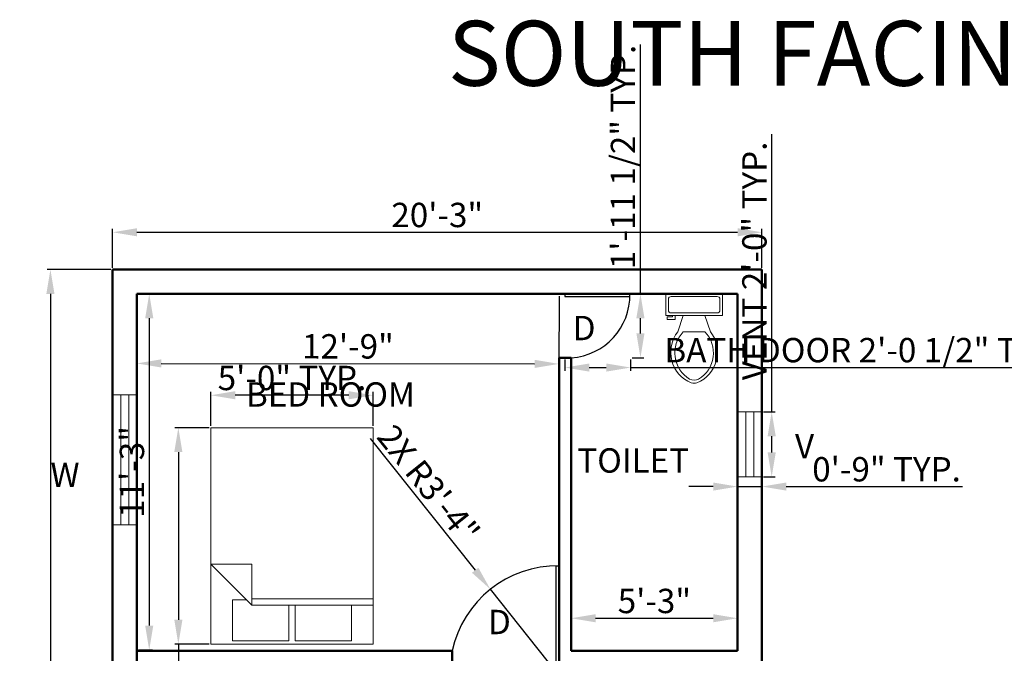
# Model space of a CAD drawing. Units: inches. Extents: x 1802 to 2621, y 1038 to 1686.
# Tile 3 of 5: x 1841 to 2205, y 1452 to 1686. Entities that reach past the tile are written whole.
import ezdxf

# ---------------------------------------------------------------- set-up
doc = ezdxf.new("R2010")
doc.units = ezdxf.units.IN
for name, color, linetype, lineweight in [('A-ANNO-DIMS', 2, 'Continuous', 18), ('A-ANNO-TEXT', 7, 'Continuous', 18), ('A-AREA-IDEN', 7, 'Continuous', 25), ('A-DOOR', 3, 'Continuous', 25), ('A-FLOR-FIXT', 9, 'Continuous', 18), ('A-FURN', 8, 'Continuous', 18), ('A-GLAZ', 4, 'Continuous', 18), ('A-WALL', 7, 'Continuous', 50)]:
    doc.layers.add(name, color=color, linetype=linetype, lineweight=lineweight)
doc.styles.get("Standard").update_dxf_attribs({"font": 'arial.ttf'})
doc.dimstyles.new('ISO-25', dxfattribs={"dimtxt": 9, "dimasz": 9, "dimexe": 1.25, "dimexo": 0.625, "dimtad": 1, "dimdec": 1, "dimrnd": 9, "dimlunit": 3, "dimtxsty": 'Standard', "dimcen": 2.5, "dimadec": 0, "dimazin": 0, "dimtfac": 1, "dimtdec": 1, "dimtmove": 0, "dimatfit": 3, "dimfxl": 1, "dimarcsym": 0})

# ---------------------------------------------------------------- blocks, each defined once
blk = doc.blocks.new('*D1')
at = {"layer": 'A-ANNO-DIMS', "color": 0, "lineweight": -2, "transparency": 16777216}
for p, q in [((1884.73, 1583.93), (1884.7, 1557.61)), ((2040.73, 1583.74), (2040.7, 1557.42)), ((1893.7, 1558.85), (2031.7, 1558.68))]:
    blk.add_line(p, q, dxfattribs=at)
at = {"layer": 'A-ANNO-DIMS', "color": 0, "transparency": 16777216}
for points in [[(1893.7, 1560.35), (1893.7, 1557.35), (1884.7, 1558.86)], [(2031.7, 1560.18), (2031.7, 1557.18), (2040.7, 1558.67)]]:
    blk.add_solid(points, dxfattribs=at)
at = {"layer": 'Defpoints', "color": 0, "transparency": 16777216}
for p in [(1884.73, 1584.56), (2040.73, 1584.37), (2040.7, 1558.67)]:
    blk.add_point(p, dxfattribs=at)
at = {"layer": 'A-ANNO-DIMS', "color": 0, "transparency": 16777216, "insert": (1962.71, 1563.99), "char_height": 9, "attachment_point": 5, "rotation": 359.9308}
blk.add_mtext('12\'-9"', dxfattribs=at)
blk = doc.blocks.new('*D2')
at = {"layer": 'A-ANNO-DIMS', "color": 0, "lineweight": -2, "transparency": 16777216}
for p, q in [((1885.35, 1584.56), (1890.53, 1584.56)), ((1889.28, 1575.56), (1889.28, 1461.93)), ((1885.35, 1452.93), (1890.53, 1452.93))]:
    blk.add_line(p, q, dxfattribs=at)
at = {"layer": 'A-ANNO-DIMS', "color": 0, "transparency": 16777216}
for points in [[(1887.78, 1575.56), (1890.78, 1575.56), (1889.28, 1584.56)], [(1887.78, 1461.93), (1890.78, 1461.93), (1889.28, 1452.93)]]:
    blk.add_solid(points, dxfattribs=at)
at = {"layer": 'Defpoints', "color": 0, "transparency": 16777216}
for p in [(1884.73, 1584.56), (1884.73, 1452.93), (1889.28, 1452.93)]:
    blk.add_point(p, dxfattribs=at)
at = {"layer": 'A-ANNO-DIMS', "color": 0, "transparency": 16777216, "insert": (1884.06, 1518.75), "char_height": 9, "attachment_point": 5, "rotation": 90}
blk.add_mtext('11\'-3"', dxfattribs=at)
blk = doc.blocks.new('*D3')
at = {"layer": 'A-ANNO-DIMS', "color": 0, "lineweight": -2, "transparency": 16777216}
for p, q in [((1875.73, 1594.18), (1875.73, 1608.58)), ((2115.73, 1594.18), (2115.73, 1608.58)), ((1884.73, 1607.33), (2106.73, 1607.33))]:
    blk.add_line(p, q, dxfattribs=at)
at = {"layer": 'A-ANNO-DIMS', "color": 0, "transparency": 16777216}
for points in [[(1884.73, 1608.83), (1884.73, 1605.83), (1875.73, 1607.33)], [(2106.73, 1608.83), (2106.73, 1605.83), (2115.73, 1607.33)]]:
    blk.add_solid(points, dxfattribs=at)
at = {"layer": 'Defpoints', "color": 0, "transparency": 16777216}
for p in [(2115.73, 1607.33), (1875.73, 1593.56), (2115.73, 1593.56)]:
    blk.add_point(p, dxfattribs=at)
at = {"layer": 'A-ANNO-DIMS', "color": 0, "transparency": 16777216, "insert": (1995.73, 1612.56), "char_height": 9, "attachment_point": 5}
blk.add_mtext('20\'-3"', dxfattribs=at)
blk = doc.blocks.new('*D4')
at = {"layer": 'A-ANNO-DIMS', "color": 0, "lineweight": -2, "transparency": 16777216}
for p, q in [((1875.1, 1593.56), (1851.51, 1593.56)), ((1852.76, 1584.56), (1852.76, 1122.56)), ((1875.1, 1113.56), (1851.51, 1113.56))]:
    blk.add_line(p, q, dxfattribs=at)
at = {"layer": 'A-ANNO-DIMS', "color": 0, "transparency": 16777216}
for points in [[(1851.26, 1584.56), (1854.26, 1584.56), (1852.76, 1593.56)], [(1851.26, 1122.56), (1854.26, 1122.56), (1852.76, 1113.56)]]:
    blk.add_solid(points, dxfattribs=at)
at = {"layer": 'Defpoints', "color": 0, "transparency": 16777216}
for p in [(1875.73, 1593.56), (1852.76, 1113.56), (1875.73, 1113.56)]:
    blk.add_point(p, dxfattribs=at)
at = {"layer": 'A-ANNO-DIMS', "color": 0, "transparency": 16777216, "insert": (1847.54, 1353.56), "char_height": 9, "attachment_point": 5, "rotation": 90}
blk.add_mtext('39\'-9"', dxfattribs=at)
blk = doc.blocks.new('*D5')
at = {"layer": 'A-ANNO-DIMS', "color": 0, "lineweight": -2, "transparency": 16777216}
for p, q in [((2045.23, 1453.18), (2045.23, 1465.91)), ((2054.23, 1464.66), (2097.73, 1464.66)), ((2106.73, 1453.18), (2106.73, 1465.91))]:
    blk.add_line(p, q, dxfattribs=at)
at = {"layer": 'A-ANNO-DIMS', "color": 0, "transparency": 16777216}
for points in [[(2054.23, 1466.16), (2054.23, 1463.16), (2045.23, 1464.66)], [(2097.73, 1466.16), (2097.73, 1463.16), (2106.73, 1464.66)]]:
    blk.add_solid(points, dxfattribs=at)
at = {"layer": 'Defpoints', "color": 0, "transparency": 16777216}
for p in [(2106.73, 1464.66), (2045.23, 1452.56), (2106.73, 1452.56)]:
    blk.add_point(p, dxfattribs=at)
at = {"layer": 'A-ANNO-DIMS', "color": 0, "transparency": 16777216, "insert": (2075.98, 1469.88), "char_height": 9, "attachment_point": 5}
blk.add_mtext('5\'-3"', dxfattribs=at)
blk = doc.blocks.new('Bed - Queen')
for p, q in [((0, -80.00003), (0, 0)), ((0, 0), (59.99999, 0)), ((59.99999, 0), (59.99999, -80.00003)), ((7.99999, -1.2), (28.79998, -1.2)), ((7.99999, -14.4), (7.99999, -1.2)), ((28.79998, -1.2), (28.79998, -14.4)), ((31.19999, -1.2), (51.99999, -1.2)), ((31.19999, -14.4), (31.19999, -1.2)), ((51.99999, -1.2), (51.99999, -16.4)), ((0, -14.4), (44.8, -14.4)), ((59.99999, -29.6), (44.8, -14.4)), ((44.8, -14.4), (44.8, -29.6)), ((44.8, -16.8), (0, -16.8)), ((51.99999, -16.4), (46.79936, -16.4)), ((44.8, -29.6), (59.99999, -29.6)), ((59.99999, -80.00003), (0, -80.00003))]:
    blk.add_line(p, q)
blk = doc.blocks.new('Toilet - top')
for p, q in [((9.5, -6), (9.5, -2)), ((-10, -8.5), (-8, -8.5)), ((-10, -9.5), (-10, -8.5)), ((-7, -9.5), (-10, -9.5)), ((-8, -8.5), (-8, -8)), ((-7, -8), (-7, -9.5)), ((-4, -8), (-6, -14)), ((4, -8), (6, -14)), ((4, -14), (-4, -14))]:
    blk.add_line(p, q)
blk.add_lwpolyline([(10.5, -8), (10.5, 0), (-10.5, 0), (-10.5, -8)], close=True)
for points in [[(-9.5, -2), (-9.5, -6)], [(8.5, -1), (-8.5, -1)], [(-8.5, -7), (8.5, -7)]]:
    blk.add_lwpolyline(points)
for centre, radius, start, end in [((-8.62, -1.88), 0.884, 81.8699, 188.1301), ((8.62, -1.88), 0.884, 351.8699, 98.1301), ((-8.62, -6.12), 0.884, 171.8699, 278.1301), ((8.62, -6.12), 0.884, 261.8699, 8.1301), ((3.52, -21.58), 12.17, 141.4691, 247.9714), ((4.2, -21.82), 11.33, 136.3677, 238.9468), ((-3.52, -21.58), 12.17, 292.0284, 38.5307), ((-4.2, -21.82), 11.33, 301.053, 43.6321), ((0, -27.88), 4, 245.7318, 294.2682), ((0, -29), 4, 254.8605, 285.1395)]:
    blk.add_arc(centre, radius, start, end)
blk = doc.blocks.new('WIN-48IN')
for p, q in [((9, 48), (0, 48)), ((3, 48), (3, 0)), ((6, 48), (6, 0)), ((9, 0), (0, 0))]:
    blk.add_line(p, q)
blk = doc.blocks.new('VENT-24IN')
for p, q in [((0, 24), (9, 24)), ((3, 0), (3, 24)), ((6, 0), (6, 24)), ((0, 0), (9, 0))]:
    blk.add_line(p, q)
blk = doc.blocks.new('DOOR-BATH-REAR-24IN')
for p, q in [((0, 23.6), (0, 22.6)), ((0, 22.6), (24, 22.6)), ((24, 22.6), (24, 23.6))]:
    blk.add_line(p, q)
blk.add_arc((0.86, 23.1), 23.15, 273.6095, 1.2378)
blk = doc.blocks.new('DOOR-BEDROOM-36IN')
for p, q in [((38.47, 0), (38.47, 36)), ((38.47, 36), (39.47, 36)), ((39.47, 0), (38.47, 0))]:
    blk.add_line(p, q)
blk.add_arc((38.97, -3.86), 39.86, 89.2813, 167.8967)
blk = doc.blocks.new('*D39')
at = {"layer": 'A-ANNO-DIMS', "color": 0, "lineweight": -2, "transparency": 16777216}
for p, q in [((2119.33, 1540.93), (2119.33, 1643.54)), ((2116.35, 1540.93), (2120.58, 1540.93)), ((2119.33, 1525.93), (2119.33, 1531.93)), ((2116.35, 1516.93), (2120.58, 1516.93))]:
    blk.add_line(p, q, dxfattribs=at)
at = {"layer": 'A-ANNO-DIMS', "color": 0, "transparency": 16777216}
for points in [[(2117.83, 1531.93), (2120.83, 1531.93), (2119.33, 1540.93)], [(2117.83, 1525.93), (2120.83, 1525.93), (2119.33, 1516.93)]]:
    blk.add_solid(points, dxfattribs=at)
at = {"layer": 'Defpoints', "color": 0, "transparency": 16777216}
for p in [(2115.73, 1540.93), (2119.33, 1540.93), (2115.73, 1516.93)]:
    blk.add_point(p, dxfattribs=at)
at = {"layer": 'A-ANNO-DIMS', "color": 0, "transparency": 16777216, "insert": (2114.11, 1596.74), "char_height": 9, "attachment_point": 5, "rotation": 90}
blk.add_mtext('VENT 2\'-0" TYP.', dxfattribs=at)
blk = doc.blocks.new('*D40')
at = {"layer": 'A-ANNO-DIMS', "color": 0, "lineweight": -2, "transparency": 16777216}
for p, q in [((2106.73, 1516.31), (2106.73, 1512.08)), ((2115.73, 1516.31), (2115.73, 1512.08)), ((2097.73, 1513.33), (2088.73, 1513.33)), ((2106.73, 1513.33), (2115.73, 1513.33)), ((2124.73, 1513.33), (2189.84, 1513.33))]:
    blk.add_line(p, q, dxfattribs=at)
at = {"layer": 'A-ANNO-DIMS', "color": 0, "transparency": 16777216}
for points in [[(2097.73, 1514.83), (2097.73, 1511.83), (2106.73, 1513.33)], [(2124.73, 1514.83), (2124.73, 1511.83), (2115.73, 1513.33)]]:
    blk.add_solid(points, dxfattribs=at)
at = {"layer": 'Defpoints', "color": 0, "transparency": 16777216}
for p in [(2106.73, 1516.93), (2115.73, 1516.93), (2115.73, 1513.33)]:
    blk.add_point(p, dxfattribs=at)
at = {"layer": 'A-ANNO-DIMS', "color": 0, "transparency": 16777216, "insert": (2161.78, 1518.56), "char_height": 9, "attachment_point": 5}
blk.add_mtext('0\'-9" TYP.', dxfattribs=at)
blk = doc.blocks.new('*D43')
at = {"layer": 'A-ANNO-DIMS', "color": 0, "lineweight": -2, "transparency": 16777216}
for p, q in [((1911.42, 1535.09), (1898.79, 1535.09)), ((1900.04, 1526.09), (1900.04, 1464.09)), ((1911.42, 1455.09), (1898.79, 1455.09)), ((1900.04, 1455.09), (1900.04, 1312.45))]:
    blk.add_line(p, q, dxfattribs=at)
at = {"layer": 'A-ANNO-DIMS', "color": 0, "transparency": 16777216}
for points in [[(1898.54, 1526.09), (1901.54, 1526.09), (1900.04, 1535.09)], [(1898.54, 1464.09), (1901.54, 1464.09), (1900.04, 1455.09)]]:
    blk.add_solid(points, dxfattribs=at)
at = {"layer": 'Defpoints', "color": 0, "transparency": 16777216}
for p in [(1912.04, 1535.09), (1900.04, 1455.09), (1912.04, 1455.09)]:
    blk.add_point(p, dxfattribs=at)
at = {"layer": 'A-ANNO-DIMS', "color": 0, "transparency": 16777216, "insert": (1894.49, 1379.27), "char_height": 9, "attachment_point": 5, "rotation": 90}
blk.add_mtext('QUEEN BED 6\'-8" TYP.', dxfattribs=at)
blk = doc.blocks.new('*D44')
at = {"layer": 'A-ANNO-DIMS', "color": 0, "lineweight": -2, "transparency": 16777216}
for p, q in [((1912.04, 1535.72), (1912.04, 1548.34)), ((1963.04, 1547.09), (1921.04, 1547.09)), ((1972.04, 1535.72), (1972.04, 1548.34))]:
    blk.add_line(p, q, dxfattribs=at)
at = {"layer": 'A-ANNO-DIMS', "color": 0, "transparency": 16777216}
for points in [[(1921.04, 1548.59), (1921.04, 1545.59), (1912.04, 1547.09)], [(1963.04, 1548.59), (1963.04, 1545.59), (1972.04, 1547.09)]]:
    blk.add_solid(points, dxfattribs=at)
at = {"layer": 'Defpoints', "color": 0, "transparency": 16777216}
for p in [(1912.04, 1547.09), (1912.04, 1535.09), (1972.04, 1535.09)]:
    blk.add_point(p, dxfattribs=at)
at = {"layer": 'A-ANNO-DIMS', "color": 0, "transparency": 16777216, "insert": (1942.04, 1552.31), "char_height": 9, "attachment_point": 5}
blk.add_mtext('5\'-0" TYP.', dxfattribs=at)
blk = doc.blocks.new('*D49')
at = {"layer": 'A-ANNO-DIMS', "color": 0, "lineweight": -2, "transparency": 16777216}
for p, q in [((2042.91, 1560.33), (2042.91, 1556.07)), ((2067.18, 1560.33), (2067.18, 1556.07)), ((2051.91, 1557.32), (2058.18, 1557.32)), ((2067.18, 1557.32), (2231.1, 1557.32))]:
    blk.add_line(p, q, dxfattribs=at)
at = {"layer": 'A-ANNO-DIMS', "color": 0, "transparency": 16777216}
for points in [[(2051.91, 1558.82), (2051.91, 1555.82), (2042.91, 1557.32)], [(2058.18, 1558.82), (2058.18, 1555.82), (2067.18, 1557.32)]]:
    blk.add_solid(points, dxfattribs=at)
at = {"layer": 'Defpoints', "color": 0, "transparency": 16777216}
for p in [(2042.91, 1560.96), (2067.18, 1560.96), (2067.18, 1557.32)]:
    blk.add_point(p, dxfattribs=at)
at = {"layer": 'A-ANNO-DIMS', "color": 0, "transparency": 16777216, "insert": (2153.64, 1562.6), "char_height": 9, "attachment_point": 5}
blk.add_mtext('BATH DOOR 2\'-0 1/2" TYP.', dxfattribs=at)
blk = doc.blocks.new('*D50')
at = {"layer": 'A-ANNO-DIMS', "color": 0, "lineweight": -2, "transparency": 16777216}
for p, q in [((2070.82, 1584.56), (2070.82, 1676.78)), ((2067.81, 1584.56), (2072.07, 1584.56)), ((2070.82, 1569.96), (2070.82, 1575.56)), ((2067.81, 1560.96), (2072.07, 1560.96))]:
    blk.add_line(p, q, dxfattribs=at)
at = {"layer": 'A-ANNO-DIMS', "color": 0, "transparency": 16777216}
for points in [[(2069.32, 1575.56), (2072.32, 1575.56), (2070.82, 1584.56)], [(2069.32, 1569.96), (2072.32, 1569.96), (2070.82, 1560.96)]]:
    blk.add_solid(points, dxfattribs=at)
at = {"layer": 'Defpoints', "color": 0, "transparency": 16777216}
for p in [(2067.18, 1584.56), (2070.82, 1584.56), (2067.18, 1560.96)]:
    blk.add_point(p, dxfattribs=at)
at = {"layer": 'A-ANNO-DIMS', "color": 0, "transparency": 16777216, "insert": (2065.54, 1635.17), "char_height": 9, "attachment_point": 5, "rotation": 90}
blk.add_mtext('1\'-11 1/2" TYP.', dxfattribs=at)
blk = doc.blocks.new('*D81')
at = {"layer": 'A-ANNO-DIMS', "color": 0, "lineweight": -2, "transparency": 16777216}
for p, q in [((1970.91, 1531.07), (2009.75, 1482.39)), ((2040.23, 1444.2), (2015.37, 1475.36))]:
    blk.add_line(p, q, dxfattribs=at)
at = {"layer": 'A-ANNO-DIMS', "color": 0, "transparency": 16777216}
blk.add_solid([(2010.93, 1483.33), (2008.58, 1481.46), (2015.37, 1475.36)], dxfattribs=at)
at = {"layer": 'Defpoints', "color": 0, "transparency": 16777216}
for p in [(2015.37, 1475.36), (2040.23, 1444.2)]:
    blk.add_point(p, dxfattribs=at)
at = {"layer": 'A-ANNO-DIMS', "color": 0, "transparency": 16777216, "insert": (1991.61, 1513.51), "char_height": 9, "attachment_point": 5, "rotation": 308.5892}
blk.add_mtext('2X R3\'-4"', dxfattribs=at)

msp = doc.modelspace()

# ---------------------------------------------------------------- linework, layer by layer
at = {"layer": 'A-WALL'}
for p, q in [((2115.73, 1593.56), (1875.73, 1593.56)), ((1875.73, 1593.56), (1875.73, 1113.56)), ((2115.73, 1113.56), (2115.73, 1593.56)), ((2106.73, 1584.56), (1884.73, 1584.56)), ((1884.73, 1584.56), (1884.73, 1346.06)), ((2106.73, 1452.56), (2106.73, 1584.56)), ((2040.73, 1560.96), (2040.73, 1378.46)), ((2040.73, 1560.96), (2045.23, 1560.96)), ((2045.23, 1560.96), (2045.23, 1452.56)), ((2001.26, 1452.56), (1884.73, 1452.56)), ((2001.26, 1452.56), (2001.26, 1448.06)), ((2106.73, 1452.56), (2045.23, 1452.56))]:
    msp.add_line(p, q, dxfattribs=at)

# ---------------------------------------------------------------- block references
at = {"layer": 'A-DOOR'}
for name, p in [('DOOR-BATH-REAR-24IN', (2042.91, 1560.96)), ('DOOR-BEDROOM-36IN', (2001.26, 1448.06))]:
    msp.add_blockref(name, p, dxfattribs=at)
at = {"layer": 'A-FLOR-FIXT'}
msp.add_blockref('Toilet - top', (2090.66, 1584.56), dxfattribs=at)
at = {"layer": 'A-FURN', "rotation": 180}
msp.add_blockref('Bed - Queen', (1972.04, 1455.09), dxfattribs=at)
at = {"layer": 'A-GLAZ'}
for name, p in [('WIN-48IN', (1875.73, 1499.22)), ('VENT-24IN', (2106.73, 1516.93))]:
    msp.add_blockref(name, p, dxfattribs=at)

# ---------------------------------------------------------------- texts
at = {"layer": 'A-ANNO-TEXT', "attachment_point": 1}
for s, width, insert, char_height in [('SOUTH FACING HOUSE', 491.7378, (1999.67, 1685.48), 24), ('D ', 17.1074, (2045.79, 1576.43), 9), ('V', 21.5258, (2127.94, 1532.78), 9), ('W', 30.0361, (1852.76, 1522.22), 9), ('D ', 17.1074, (2014.48, 1467.77), 9)]:
    msp.add_mtext_dynamic_manual_height_columns(s, width=width, gutter_width=12.5, heights=[0], dxfattribs=dict(at, insert=insert, char_height=char_height))
at = {"layer": 'A-AREA-IDEN', "char_height": 9, "attachment_point": 1}
for s, insert in [('BED ROOM', (1925.02, 1551.87)), ('TOILET', (2047.49, 1527.48))]:
    msp.add_mtext_dynamic_manual_height_columns(s, width=82.6611, gutter_width=12.5, heights=[0], dxfattribs=dict(at, insert=insert))

# ---------------------------------------------------------------- dimensions: what is measured, and where the dimension line sits
at = {"layer": 'A-ANNO-DIMS'}
for base, p1, p2, angle, text, picture, middle in [((2070.82, 1584.56), (2067.18, 1560.96), (2067.18, 1584.56), 90, '<> TYP.', '*D50', (2065.54, 1635.17)), ((2119.33, 1540.93), (2115.73, 1516.93), (2115.73, 1540.93), 90, 'VENT <> TYP.', '*D39', (2114.11, 1596.74)), ((1912.04, 1547.09), (1972.04, 1535.09), (1912.04, 1535.09), 180, '<> TYP.', '*D44', (1942.04, 1552.31)), ((1900.04, 1455.09), (1912.04, 1535.09), (1912.04, 1455.09), 270, 'QUEEN BED <> TYP.', '*D43', (1894.49, 1379.27))]:
    dim = msp.add_linear_dim(base=base, p1=p1, p2=p2, angle=angle, text=text, dimstyle='ISO-25', override={"dimdec": 1, "dimlfac": 1, "dimrnd": 0, "dimzin": 1, "dimdsep": 46, "dimlunit": 4, "dimfrac": 2}, dxfattribs=at)
    dim.commit()
    dim.dimension.update_dxf_attribs({"geometry": picture, "text_midpoint": middle})
for base, p1, p2, picture, middle in [((2115.73, 1607.33), (1875.73, 1593.56), (2115.73, 1593.56), '*D3', (1995.73, 1612.56)), ((2106.73, 1464.66), (2045.23, 1452.56), (2106.73, 1452.56), '*D5', (2075.98, 1469.88))]:
    dim = msp.add_linear_dim(base=base, p1=p1, p2=p2, dimstyle='ISO-25', override={"dimclrd": 0, "dimclre": 0, "dimclrt": 0}, dxfattribs=at)
    dim.commit()
    dim.dimension.update_dxf_attribs({"geometry": picture, "text_midpoint": middle})
for base, p1, p2, text, picture, middle in [((2067.18, 1557.32), (2042.91, 1560.96), (2067.18, 1560.96), 'BATH DOOR <> TYP.', '*D49', (2153.64, 1562.6)), ((2115.73, 1513.33), (2106.73, 1516.93), (2115.73, 1516.93), '<> TYP.', '*D40', (2161.78, 1518.56))]:
    dim = msp.add_linear_dim(base=base, p1=p1, p2=p2, text=text, dimstyle='ISO-25', override={"dimdec": 1, "dimlfac": 1, "dimrnd": 0, "dimzin": 1, "dimdsep": 46, "dimlunit": 4, "dimfrac": 2}, dxfattribs=at)
    dim.commit()
    dim.dimension.update_dxf_attribs({"geometry": picture, "text_midpoint": middle})
for base, p1, p2, picture, middle in [((1852.76, 1113.56), (1875.73, 1593.56), (1875.73, 1113.56), '*D4', (1847.54, 1353.56)), ((1889.28, 1452.93), (1884.73, 1584.56), (1884.73, 1452.93), '*D2', (1884.06, 1518.75))]:
    dim = msp.add_linear_dim(base=base, p1=p1, p2=p2, angle=90, dimstyle='ISO-25', override={"dimclrd": 0, "dimclre": 0, "dimclrt": 0}, dxfattribs=at)
    dim.commit()
    dim.dimension.update_dxf_attribs({"geometry": picture, "text_midpoint": middle})
dim = msp.add_aligned_dim(p1=(1884.73, 1584.56), p2=(2040.73, 1584.37), distance=-25.7, dimstyle='ISO-25', override={"dimclrd": 0, "dimclre": 0, "dimclrt": 0}, dxfattribs=at)
dim.commit()
dim.dimension.update_dxf_attribs({"geometry": '*D1', "text_midpoint": (1962.71, 1563.99)})
dim = msp.add_radius_dim(center=(2040.23, 1444.2), mpoint=(2015.37, 1475.36), text='2X <>', dimstyle='ISO-25', override={"dimdec": 1, "dimlfac": 1, "dimrnd": 0, "dimzin": 1, "dimdsep": 46, "dimlunit": 4, "dimfrac": 2}, dxfattribs=at)
dim.commit()
dim.dimension.update_dxf_attribs({"geometry": '*D81', "text_midpoint": (1991.61, 1513.51)})

doc.saveas('drawing.dxf')
